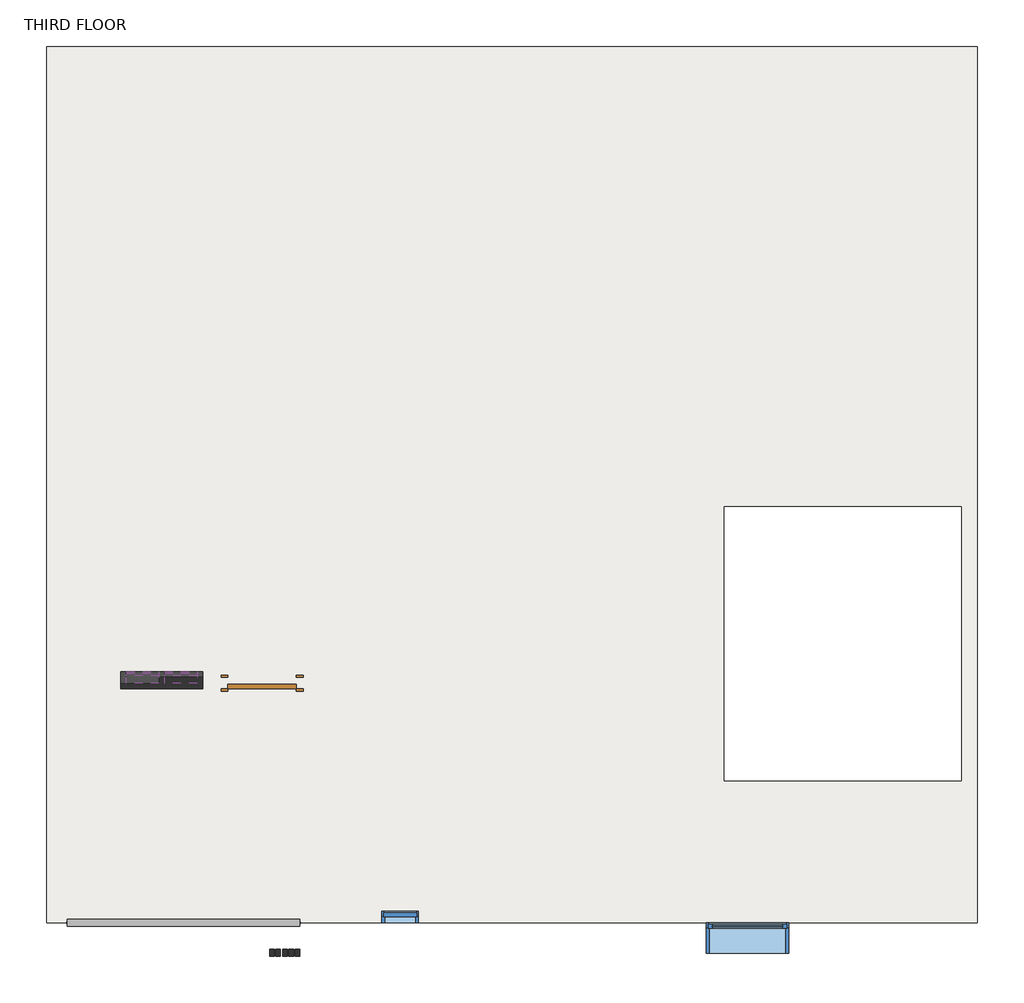
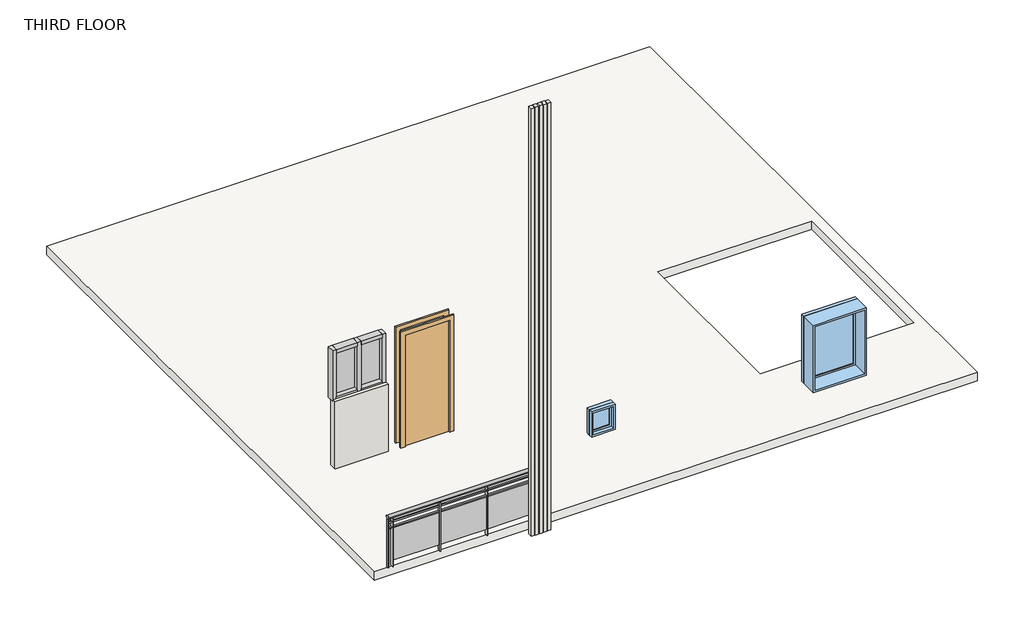
# One storey: 7 members, 2 plates, 2 walls, 2 windows, 1 door, 1 railing, 1 slab.
"""IFC4 building model written with IfcOpenShell, lengths in millimetres."""

from ifc_helpers import new_model, si_unit, point, frame, origin, place, context, project, spatial, polyline, ellipse_curve, trimmed, outline, extrude, transform, mapped, element, save
from ifc_brep_helpers import plane_surface, extruded_surface, advanced_brep
from components import door_e00f436c, member_d959a85f, member_843225dc, member_54f829b7, system_panel_glazed_8fc33089, walls_7_walls_7_9077e6f4, fixed_bw_be0fa6e9, fixed_ven_0bde2124

model = new_model("IFC4")

# Units and contexts
model_context = context("Model", 3, world=origin())
ifc_project = project(units=[si_unit("LENGTHUNIT", "METRE", prefix="MILLI")], contexts=[model_context])

# Site, building, storey
site = spatial("IfcSite", under=ifc_project)
building = spatial("IfcBuilding", under=site)
storey = spatial("IfcBuildingStorey", under=building, Name="THIRD FLOOR", Elevation=9144.0)

# Door
placement = place(None, origin())
door_shape = door_e00f436c(model_context)
element("IfcDoor", 1, ObjectType="Single-Flush : 36\" x 84\"", at=placement, inside=storey, context=model_context, shape_type="MappedRepresentation", body=[
    mapped(door_shape, transform((-4124.5569651, 3118.5055142, 9144.0), x_axis=(1.0, 0.0, 0.0), y_axis=(0.0, 1.0, 0.0), z_axis=(0.0, 0.0, 1.0))),
])

# Members
member_shape = member_d959a85f(model_context)
element("IfcMember", 2, ObjectType="Rectangular Mullion : 2.5\" x 5\" rectangular", at=placement, inside=storey, context=model_context, shape_type="MappedRepresentation", body=[
    mapped(member_shape, transform((-4784.9569651, 3182.0055142, 10333.4584417), x_axis=(1.0, 0.0, 0.0), y_axis=(0.0, -1.0, 0.0), z_axis=(0.0, 0.0, -1.0))),
])
element("IfcMember", 3, ObjectType="Rectangular Mullion : 2.5\" x 5\" rectangular", at=placement, inside=storey, context=model_context, shape_type="MappedRepresentation", body=[
    mapped(member_shape, transform((-5699.3569651, 3182.0055142, 11252.2), x_axis=(-1.0, 0.0, 0.0), y_axis=(0.0, -1.0, 0.0), z_axis=(0.0, 0.0, 1.0))),
])
member_2_shape = member_843225dc(model_context)
element("IfcMember", 4, ObjectType="Rectangular Mullion : 2.5\" x 5\" rectangular", at=placement, inside=storey, context=model_context, shape_type="MappedRepresentation", body=[
    mapped(member_2_shape, transform((-4848.4569651, 3182.0055142, 11252.2), x_axis=(0.0, 0.0, 1.0), y_axis=(0.0, -1.0, 0.0), z_axis=(1.0, 0.0, 0.0))),
])
element("IfcMember", 5, ObjectType="Rectangular Mullion : 2.5\" x 5\" rectangular", at=placement, inside=storey, context=model_context, shape_type="MappedRepresentation", body=[
    mapped(member_2_shape, transform((-5273.9069651, 3182.0055142, 11252.2), x_axis=(0.0, 0.0, 1.0), y_axis=(0.0, -1.0, 0.0), z_axis=(1.0, 0.0, 0.0))),
])
element("IfcMember", 6, ObjectType="Rectangular Mullion : 2.5\" x 5\" rectangular", at=placement, inside=storey, context=model_context, shape_type="MappedRepresentation", body=[
    mapped(member_2_shape, transform((-5635.8569651, 3182.0055142, 10333.4584417), x_axis=(0.0, 0.0, -1.0), y_axis=(0.0, -1.0, 0.0), z_axis=(-1.0, 0.0, 0.0))),
])
element("IfcMember", 7, ObjectType="Rectangular Mullion : 2.5\" x 5\" rectangular", at=placement, inside=storey, context=model_context, shape_type="MappedRepresentation", body=[
    mapped(member_2_shape, transform((-5210.4069651, 3182.0055142, 10333.4584417), x_axis=(0.0, 0.0, -1.0), y_axis=(0.0, -1.0, 0.0), z_axis=(-1.0, 0.0, 0.0))),
])
member_3_shape = member_54f829b7(model_context)
element("IfcMember", 8, ObjectType="Rectangular Mullion : 2.5\" x 5\" rectangular", at=placement, inside=storey, context=model_context, shape_type="MappedRepresentation", body=[
    mapped(member_3_shape, transform((-5242.1569651, 3182.0055142, 10333.4584417), x_axis=(1.0, 0.0, 0.0), y_axis=(0.0, -1.0, 0.0), z_axis=(0.0, 0.0, -1.0))),
])

# Plates
system_panel_glazed_shape = system_panel_glazed_8fc33089(model_context)
element("IfcPlate", 9, ObjectType="System Panel : Glazed", at=placement, inside=storey, context=model_context, shape_type="MappedRepresentation", body=[
    mapped(system_panel_glazed_shape, transform((-5454.8819651, 3182.0055142, 10396.9584417), x_axis=(1.0, 0.0, 0.0), y_axis=(0.0, 1.0, 0.0), z_axis=(0.0, 0.0, 1.0))),
])
element("IfcPlate", 10, ObjectType="System Panel : Glazed", at=placement, inside=storey, context=model_context, shape_type="MappedRepresentation", body=[
    mapped(system_panel_glazed_shape, transform((-5029.4319651, 3182.0055142, 10396.9584417), x_axis=(1.0, 0.0, 0.0), y_axis=(0.0, 1.0, 0.0), z_axis=(0.0, 0.0, 1.0))),
])

# Railing
element("IfcRailing", 11, ObjectType="Glass Panel - Bottom Fill", at=placement, inside=storey, context=model_context, shape_type="SolidModel", body=[
    advanced_brep(
    [(-6296.2569651, 489.6055142, 10058.4), (-6296.2569651, 413.4055142, 10058.4), (-3705.4569651, 489.6055142, 10058.4), (-3705.4569651, 413.4055142, 10058.4)],
    [
        (0, 1, ellipse_curve(frame((-6296.2569651, 451.5055142, 10058.4), z_axis=(-1.0, 0.0, 0.0), x_axis=(0.0, -1.0, 0.0)), 38.1, 28.575)),
        (1, 0, ellipse_curve(frame((-6296.2569651, 451.5055142, 10058.4), z_axis=(-1.0, 0.0, 0.0), x_axis=(0.0, -1.0, 0.0)), 38.1, 28.575)),
        (2, 3, ellipse_curve(frame((-3705.4569651, 451.5055142, 10058.4), z_axis=(1.0, 0.0, 0.0), x_axis=(0.0, -1.0, 0.0)), 38.1, 28.575)),
        (3, 2, ellipse_curve(frame((-3705.4569651, 451.5055142, 10058.4), z_axis=(1.0, 0.0, 0.0), x_axis=(0.0, -1.0, 0.0)), 38.1, 28.575)),
        (0, 2),
        (3, 1),
    ],
    [
        plane_surface(frame((-6296.2569651, 451.5055142, 10058.4), z_axis=(-1.0, 0.0, 0.0), x_axis=(0.0, 1.0, 0.0))),
        plane_surface(frame((-3705.4569651, 451.5055142, 10058.4), z_axis=(1.0, 0.0, 0.0), x_axis=(0.0, 1.0, 0.0))),
        extruded_surface(trimmed(ellipse_curve(frame((-3705.4569651, 451.5055142, 10058.4), z_axis=(-1.0, 0.0, 0.0), x_axis=(0.0, -1.0, 0.0)), 38.1, 28.575), [point((-3705.4569651, 489.6055142, 10058.4))], [point((-3705.4569651, 413.4055142, 10058.4))], True, "CARTESIAN"), (-2590.8, 0.0, 0.0), 2590.8),
        extruded_surface(trimmed(ellipse_curve(frame((-3705.4569651, 451.5055142, 10058.4), z_axis=(-1.0, 0.0, 0.0), x_axis=(0.0, -1.0, 0.0)), 38.1, 28.575), [point((-3705.4569651, 413.4055142, 10058.4))], [point((-3705.4569651, 489.6055142, 10058.4))], True, "CARTESIAN"), (-2590.8, 0.0, 0.0), 2590.8),
    ],
    [
        (0, [[1, 2]]),
        (1, [[3, 4]]),
        (2, [[-1, 5, -4, 6]]),
        (3, [[-2, -6, -3, -5]]),
    ],
),
    extrude(outline(polyline([(-6296.2569651, 438.8055142), (-6296.2569651, 464.2055142), (-3705.4569651, 464.2055142), (-3705.4569651, 438.8055142), (-6296.2569651, 438.8055142)])), frame((0.0, 0.0, 9944.1), z_axis=(0.0, 0.0, 1.0), x_axis=(1.0, 0.0, 0.0)), (0.0, 0.0, 1.0), 25.4),
    extrude(outline(polyline([(-6296.2569651, 438.8055142), (-6296.2569651, 464.2055142), (-3705.4569651, 464.2055142), (-3705.4569651, 438.8055142), (-6296.2569651, 438.8055142)])), frame((0.0, 0.0, 9842.5), z_axis=(0.0, 0.0, 1.0), x_axis=(1.0, 0.0, 0.0)), (0.0, 0.0, 1.0), 25.4),
    extrude(outline(polyline([(-3788.0069651, 426.1055142), (-3788.0069651, 476.9055142), (-3775.3069651, 476.9055142), (-3775.3069651, 426.1055142), (-3788.0069651, 426.1055142)])), frame((0.0, 0.0, 9144.0), z_axis=(0.0, 0.0, 1.0), x_axis=(1.0, 0.0, 0.0)), (0.0, 0.0, 1.0), 885.6788223),
    extrude(outline(polyline([(-4594.4569651, 458.0406712), (-3781.6569651, 458.0406712), (-3781.6569651, 451.6906712), (-4594.4569651, 451.6906712), (-4594.4569651, 458.0406712)])), frame((0.0, 0.0, 9245.6), z_axis=(0.0, 0.0, 1.0), x_axis=(1.0, 0.0, 0.0)), (0.0, 0.0, 1.0), 596.9),
    extrude(outline(polyline([(-4600.8069651, 426.1055142), (-4600.8069651, 476.9055142), (-4588.1069651, 476.9055142), (-4588.1069651, 426.1055142), (-4600.8069651, 426.1055142)])), frame((0.0, 0.0, 9144.0), z_axis=(0.0, 0.0, 1.0), x_axis=(1.0, 0.0, 0.0)), (0.0, 0.0, 1.0), 885.6788223),
    extrude(outline(polyline([(-5407.2569651, 458.0406712), (-4594.4569651, 458.0406712), (-4594.4569651, 451.6906712), (-5407.2569651, 451.6906712), (-5407.2569651, 458.0406712)])), frame((0.0, 0.0, 9245.6), z_axis=(0.0, 0.0, 1.0), x_axis=(1.0, 0.0, 0.0)), (0.0, 0.0, 1.0), 596.9),
    extrude(outline(polyline([(-5413.6069651, 426.1055142), (-5413.6069651, 476.9055142), (-5400.9069651, 476.9055142), (-5400.9069651, 426.1055142), (-5413.6069651, 426.1055142)])), frame((0.0, 0.0, 9144.0), z_axis=(0.0, 0.0, 1.0), x_axis=(1.0, 0.0, 0.0)), (0.0, 0.0, 1.0), 885.6788223),
    extrude(outline(polyline([(-6220.0569651, 458.0406712), (-5407.2569651, 458.0406712), (-5407.2569651, 451.6906712), (-6220.0569651, 451.6906712), (-6220.0569651, 458.0406712)])), frame((0.0, 0.0, 9245.6), z_axis=(0.0, 0.0, 1.0), x_axis=(1.0, 0.0, 0.0)), (0.0, 0.0, 1.0), 596.9),
    extrude(outline(polyline([(-6226.4069651, 426.1055142), (-6226.4069651, 476.9055142), (-6213.7069651, 476.9055142), (-6213.7069651, 426.1055142), (-6226.4069651, 426.1055142)])), frame((0.0, 0.0, 9144.0), z_axis=(0.0, 0.0, 1.0), x_axis=(1.0, 0.0, 0.0)), (0.0, 0.0, 1.0), 885.6788223),
    extrude(outline(polyline([(-3718.1569651, 441.9805142), (-3718.1569651, 461.0305142), (-3699.1069651, 461.0305142), (-3699.1069651, 441.9805142), (-3718.1569651, 441.9805142)])), frame((0.0, 0.0, 9144.0), z_axis=(0.0, 0.0, 1.0), x_axis=(1.0, 0.0, 0.0)), (0.0, 0.0, 1.0), 885.6788223),
    extrude(outline(polyline([(-6302.6069651, 441.9805142), (-6302.6069651, 461.0305142), (-6283.5569651, 461.0305142), (-6283.5569651, 441.9805142), (-6302.6069651, 441.9805142)])), frame((0.0, 0.0, 9144.0), z_axis=(0.0, 0.0, 1.0), x_axis=(1.0, 0.0, 0.0)), (0.0, 0.0, 1.0), 885.6788223),
])

# Slab
element("IfcSlab", 12, ObjectType="Generic - 12\"", at=placement, inside=storey, context=model_context, shape_type="SweptSolid", body=[
    extrude(outline(polyline([(3838.3430349, 10205.1055142), (3838.3430349, 451.5055142), (-6524.8569651, 451.5055142), (-6524.8569651, 10205.1055142), (3838.3430349, 10205.1055142)]), holes=[polyline([(3660.5430349, 5080.6555142), (1018.9430349, 5080.6555142), (1018.9430349, 2032.6555142), (3660.5430349, 2032.6555142), (3660.5430349, 5080.6555142)])]), frame((0.0, 0.0, 8991.6), z_axis=(0.0, 0.0, 1.0), x_axis=(1.0, 0.0, 0.0)), (0.0, 0.0, 1.0), 152.4),
])

# Walls
element("IfcWall", 13, ObjectType="5\"", at=placement, inside=storey, context=model_context, shape_type="SweptSolid", body=[
    extrude(outline(polyline([(-4784.9569651, 3055.0055142), (-5699.3569651, 3055.0055142), (-5699.3569651, 3182.0055142), (-4784.9569651, 3182.0055142), (-4784.9569651, 3055.0055142)])), frame((0.0, 0.0, 8204.2), z_axis=(0.0, 0.0, 1.0), x_axis=(1.0, 0.0, 0.0)), (0.0, 0.0, 1.0), 2159.0),
])
walls_7_walls_7_shape = walls_7_walls_7_9077e6f4(model_context)
element("IfcWall", 14, ObjectType="Walls 7 : Walls 7", at=placement, inside=storey, context=model_context, shape_type="MappedRepresentation", body=[
    mapped(walls_7_walls_7_shape, transform((0.0, 0.0, 0.0), x_axis=(1.0, 0.0, 0.0), y_axis=(0.0, 1.0, 0.0), z_axis=(0.0, 0.0, 1.0))),
])

# Windows
fixed_bw_shape = fixed_bw_be0fa6e9(model_context)
element("IfcWindow", 15, ObjectType="Fixed : BW", at=placement, inside=storey, context=model_context, shape_type="MappedRepresentation", body=[
    mapped(fixed_bw_shape, transform((1316.0073388, 281.3921573, 9118.6), x_axis=(1.0, 0.0, 0.0), y_axis=(0.0, 1.0, 0.0), z_axis=(0.0, 0.0, 1.0))),
])
fixed_ven_shape = fixed_ven_0bde2124(model_context)
element("IfcWindow", 16, ObjectType="Fixed : VEN", at=placement, inside=storey, context=model_context, shape_type="MappedRepresentation", body=[
    mapped(fixed_ven_shape, transform((-2549.7569651, 515.0055142, 9369.782033), x_axis=(1.0, 0.0, 0.0), y_axis=(0.0, 1.0, 0.0), z_axis=(0.0, 0.0, 1.0))),
])

save(model, "model.ifc")

# Revit data of these elements
# Type "Single-Flush : 36\" x 84\""
#   Type Mark = "1"
#   Construction Type Id = "MDOOR"
#   Assembly Code = "C1020"
#   Analytic Construction = "Metal"
#   Thickness = 0' - 2"
#   Heat Transfer Coefficient (U) = 0.651978 BTU/(h·ft²·°F)
#   Height = 6' - 8"
#   Trim Projection Ext = 0' - 1"
#   Trim Projection Int = 0' - 1"
#   Trim Width = 0' - 3"
#   Width = 2' - 6"
#   Define Thermal Properties by = 1
#   Define Thermal Properties by = 1
#   Door Material = Door - Panel
#   Frame Material = Door - Frame
#   Visual Light Transmittance = 0
#   Solar Heat Gain Coefficient = 0
#   Function = (empty or 0)
#   Wall Closure = (empty or 0)
# Type "Rectangular Mullion : 2.5\" x 5\" rectangular"
#   built-in parameter 1007304 = 0.416667 (stored number, unit not read)
#   built-in parameter 1007301 = 0.104167 (stored number, unit not read)
#   built-in parameter 1007300 = 0.104167 (stored number, unit not read)
# Type "System Panel : Glazed"
#   Construction Type Id = "GSP4R"
#   Analytic Construction = "1/8 in Pilkington single glazing"
#   Visual Light Transmittance = 0.9
#   Solar Heat Gain Coefficient = 0.86
#   Heat Transfer Coefficient (U) = 1.18115 BTU/(h·ft²·°F)
#   Define Thermal Properties by = 1
# Type "Glass Panel - Bottom Fill"
#   Assembly Code = "C2010400"
#   built-in parameter 1008612 = 0.0416667 (stored number, unit not read)
#   built-in parameter 1008611 = 0.0416667 (stored number, unit not read)
#   built-in parameter 1008609 = 0.333333 (stored number, unit not read)
#   built-in parameter 1008604 = 0.166667 (stored number, unit not read)
#   built-in parameter 1008603 = 0.166667 (stored number, unit not read)
#   Railing Height = 3' - 0"
#   built-in parameter 1008630 = 2
#   built-in parameter 1008610 = 2
#   built-in parameter 1008618 = Baluster - Square : 3/4"
# Type "Generic - 12\""
#   Assembly Code = "B1010"
#   Function = 0
#   Layers, outside or top first: 0' - 6" no material (function 1)
# Type "5\""
#   Assembly Code = "B2010"
#   Layers, outside or top first: 0' - 5" "Concrete Masonry Units" (function 1)
# Type "Fixed : BW"
#   Type Mark = "18"
#   Construction Type Id = "GSP4R"
#   Assembly Code = "B2020100"
#   Analytic Construction = "1/8 in Pilkington single glazing"
#   Visual Light Transmittance = 0.9
#   Solar Heat Gain Coefficient = 0.78
#   Heat Transfer Coefficient (U) = 0.6496 BTU/(h·ft²·°F)
#   Height = 4' - 0"
#   Default Sill Height = 3' - 0"
#   Width = 3' - 0"
#   Window Inset = 0' - 0 3/4"
#   Define Thermal Properties by = 1
#   Glass Pane Material = Glass
#   Sash Material = Sash
#   Wall Closure = (empty or 0)
# Type "Fixed : VEN"
#   Type Mark = "19"
#   Construction Type Id = "GSP4R"
#   Assembly Code = "B2020100"
#   Analytic Construction = "1/8 in Pilkington single glazing"
#   Visual Light Transmittance = 0.9
#   Solar Heat Gain Coefficient = 0.78
#   Heat Transfer Coefficient (U) = 0.6496 BTU/(h·ft²·°F)
#   Height = 1' - 6"
#   Default Sill Height = 3' - 0"
#   Width = 1' - 4"
#   Window Inset = 0' - 0 3/4"
#   Define Thermal Properties by = 1
#   Glass Pane Material = Glass
#   Sash Material = Sash
#   Wall Closure = (empty or 0)
# Element 1 (IfcDoor, "Single-Flush : 36\" x 84\"")
#   Phase Created = New Construction
#   Materials on its faces: "Door - Frame", "Door - Panel"
# Elements 2, 3, 4, 5, 6, 7, 8 (IfcMember, "Rectangular Mullion : 2.5\" x 5\" rectangular")
#   Phase Created = New Construction
#   Materials on its faces: "Aluminum"
# Elements 9, 10 (IfcPlate, "System Panel : Glazed")
#   Phase Created = New Construction
#   Materials on its faces: "Glass"
# Element 11 (IfcRailing, "Glass Panel - Bottom Fill")
#   Phase Created = New Construction
#   Materials on its faces: "Glass"
# Element 12 (IfcSlab, "Generic - 12\"")
#   Height Offset From Level = 0' - 0"
#   Phase Created = New Construction
#   Materials on its faces: "Default Floor", "1 wall brown"
# Element 13 (IfcWall, "5\"")
#   built-in parameter 1001111 = -3' - 1"
#   Top Offset = 0' - 0"
#   Base Offset = -3' - 1"
#   Unconnected Height = 7' - 1"
#   wall height = 7' - 1"
#   Phase Created = New Construction
#   Base Constraint = THIRD FLOOR
#   Materials on its faces: "Concrete Masonry Units", "1 wall white"
# Element 14 (IfcWall, "Walls 7 : Walls 7")
#   Phase Created = New Construction
#   Materials on its faces: "1 wood", "Default Wall"
# Element 15 (IfcWindow, "Fixed : BW")
#   Mark = "9"
#   Phase Created = New Construction
#   Materials on its faces: "Sash", "Glass"
# Element 16 (IfcWindow, "Fixed : VEN")
#   Mark = "12"
#   Phase Created = New Construction
#   Materials on its faces: "Sash", "Glass"
# Materials
#   "Door - Panel": class "Wood", colour RGB 210 159 95, transparency 0, Cost = 0
#   "Door - Frame": colour RGB 118 70 51, transparency 0, Cost = 0
#   "Concrete Masonry Units": class "Masonry", colour RGB 227 227 227, transparency 0, Description = "Concrete masonry units", Cost = 0
#   "Glass": class "Glass", colour RGB 0 128 192, transparency 0.75, Description = "Soda Lime Glass", Cost = 0
#   "Sash": class "Wood", colour RGB 224 178 126, transparency 0, Cost = 0
#   "Aluminum": class "Metal", colour RGB 247 247 247, transparency 0, Description = "Aluminum 6061", Cost = 0
#   "Default Floor": colour RGB 128 128 128, transparency 0, Cost = 0
#   "1 wall brown": class "Generic", colour RGB 61 46 37, transparency 0, Cost = 0
#   "1 wall white": class "Generic", colour RGB 244 245 241, transparency 0, Cost = 0
#   "1 wood": class "Generic", colour RGB 120 120 120, transparency 0, Cost = 0
#   "Default Wall": colour RGB 128 128 128, transparency 0, Cost = 0
